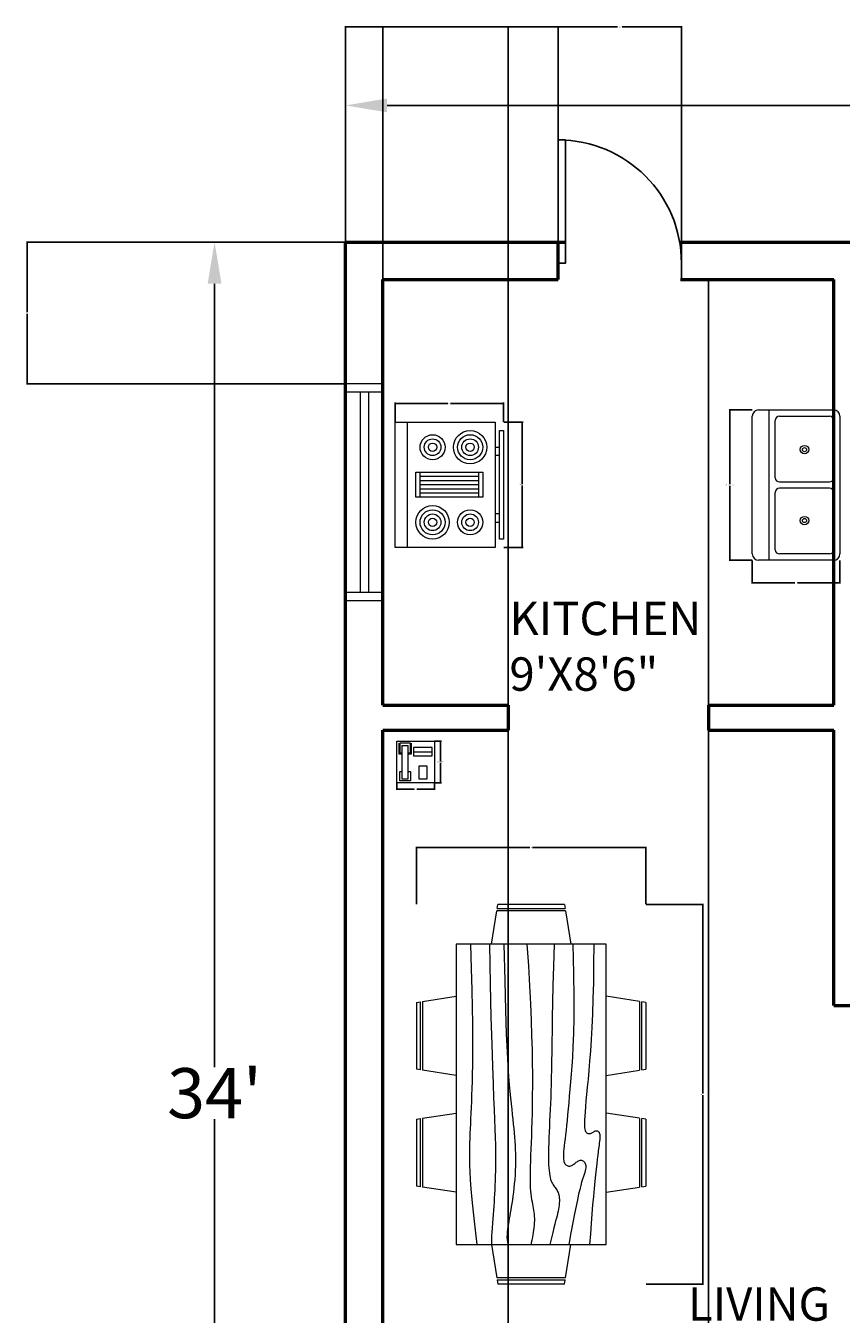
# Model space of a CAD drawing. Units: inches. Extents: x 177 to 602, y 30 to 608.
# Tile 3 of 4: x 177 to 372, y 299 to 608. Entities that reach past the tile are written whole.
import ezdxf

# ---------------------------------------------------------------- set-up
doc = ezdxf.new("R2010")
doc.units = ezdxf.units.IN
doc.header["$MEASUREMENT"] = 0
for name, color, linetype, lineweight in [('A-ANNO-DIMS', 2, 'Continuous', 18), ('A-AREA-IDEN', 7, 'Continuous', 25), ('A-DOOR', 3, 'Continuous', 25), ('A-EQPM', 9, 'Continuous', 18), ('A-FLOR-CASE', 32, 'Continuous', 25), ('A-FLOR-FIXT', 9, 'Continuous', 20), ('A-FURN', 8, 'Continuous', 18), ('A-GLAZ', 4, 'Continuous', 18), ('A-WALL', 7, 'Continuous', 50)]:
    doc.layers.add(name, color=color, linetype=linetype, lineweight=lineweight)
doc.styles.get("Standard").update_dxf_attribs({"font": 'arial.ttf'})
doc.dimstyles.get("Standard").update_dxf_attribs({"dimtxt": 0.18, "dimasz": 0.18, "dimexe": 0.18, "dimexo": 0.0625, "dimgap": 0.09, "dimtad": 0, "dimtih": 1, "dimtoh": 1, "dimdec": 1, "dimzin": 0, "dimdsep": 46, "dimlunit": 4, "dimtxsty": 'Standard', "dimcen": 0.09, "dimadec": 0, "dimazin": 0, "dimtfac": 1, "dimtdec": 1, "dimtofl": 0, "dimtmove": 0, "dimatfit": 3, "dimfxl": 1, "dimtolj": 1, "dimtzin": 0, "dimarcsym": 0})

# ---------------------------------------------------------------- blocks, each defined once
blk = doc.blocks.new('*U2')
for p, q in [((0, 0), (0, -100)), ((750, 0), (750, -100))]:
    blk.add_line(p, q)
blk.add_lwpolyline([(0, 0), (0, 750), (43.75, 750), (43.75, 0)], close=True)
blk.add_arc((0, 0), 750, 0, 90)
blk = doc.blocks.new('Range-Oven - 30 in top')
for p, q in [((0, -3), (30, -3)), ((12, -6), (18, -6)), ((13, -20), (13, -6)), ((14, -6), (14, -20)), ((15, -20), (15, -6)), ((16, -6), (16, -20)), ((17, -20), (17, -6)), ((18, -20), (12, -20)), ((6, -24), (6, -25)), ((8, -25), (8, -24)), ((22, -25), (22, -24)), ((24, -24), (24, -25))]:
    blk.add_line(p, q)
for points in [[(0, -24), (0, 0), (30, 0), (30, -24)], [(12, -21), (12, -5), (18, -5), (18, -21)], [(2, -26), (2, -25), (28, -25), (28, -26)]]:
    blk.add_lwpolyline(points, close=True)
for centre, radius in [((6, -9), 4), ((6, -9), 3), ((24, -9), 3), ((6, -9), 2), ((6, -9), 1), ((24, -9), 2), ((24, -9), 1), ((6, -18), 3), ((24, -18), 4), ((24, -18), 3), ((6, -18), 2), ((6, -18), 1), ((24, -18), 2), ((24, -18), 1)]:
    blk.add_circle(centre, radius)
blk = doc.blocks.new('Sink-double - 36 in top')
for p, q in [((-18, -4), (18, -4)), ((-0.75, -18.5), (-0.75, -6.5)), ((0.75, -6.5), (0.75, -18.5))]:
    blk.add_line(p, q)
for points in [[(-16.5, 0), (16.5, 0)], [(-18, -19.5), (-18, -1.5)], [(18, -1.5), (18, -19.5)], [(-15.5, -5.5), (-1.75, -5.5)], [(1.75, -5.5), (15.5, -5.5)], [(-16.5, -18.5), (-16.5, -6.5)], [(16.5, -6.5), (16.5, -18.5)], [(16.5, -21), (-16.5, -21)], [(-1.75, -19.5), (-15.5, -19.5)], [(15.5, -19.5), (1.75, -19.5)]]:
    blk.add_lwpolyline(points)
for centre, radius in [((-8.5, -12.5), 1), ((-8.5, -12.5), 0.5), ((8.5, -12.5), 1), ((8.5, -12.5), 0.5)]:
    blk.add_circle(centre, radius)
for centre, radius, start, end in [((-16.5, -1.5), 1.5, 90, 180), ((16.5, -1.5), 1.5, 0, 90), ((-15.5, -6.5), 1, 90, 180), ((-1.75, -6.5), 1, 0, 90), ((1.75, -6.5), 1, 90, 180), ((15.5, -6.5), 1, 0, 90), ((-15.5, -18.5), 1, 180, 270), ((-1.75, -18.5), 1, 270, 0), ((1.75, -18.5), 1, 180, 270), ((15.5, -18.5), 1, 270, 0), ((-16.5, -19.5), 1.5, 180, 270), ((16.5, -19.5), 1.5, 270, 0)]:
    blk.add_arc(centre, radius, start, end)
blk = doc.blocks.new('Dining Set - 36 x 72 in.')
for p, q in [((-22.2343, 26.00059), (-23.4847, 17.99762)), ((-22.2304, 26), (-5.7608, 26)), ((-22, 27.5), (-22.1562, 26.50042)), ((-5.8416, 26.5), (-22.1534, 26.5)), ((-22, 27.5), (-6, 27.5)), ((-5.8437, 26.49966), (-6, 27.5)), ((-4.5152, 17.99762), (-5.7655, 25.99926)), ((5.7657, 26.00059), (4.5153, 17.99762)), ((5.7696, 26), (22.2392, 26)), ((6, 27.5), (5.8438, 26.50042)), ((22.1584, 26.5), (5.8466, 26.5)), ((6, 27.5), (22, 27.5)), ((22.1563, 26.49966), (22, 27.5)), ((23.4848, 17.99762), (22.2345, 25.99926)), ((36, 18), (-36, 18)), ((-36, 18), (-36, -18)), ((36, -18), (36, 18)), ((-44.0006, 8.23428), (-35.9976, 9.48474)), ((44.0006, 8.23428), (35.9976, 9.48474)), ((-45.5, 8), (-44.5004, 8.15617)), ((-45.5, 8), (-45.5, -8)), ((-44.5, -8.15843), (-44.5, 8.15338)), ((-44, 8.23041), (-44, -8.23915)), ((44, 8.23041), (44, -8.23915)), ((44.5, -8.15843), (44.5, 8.15338)), ((45.5, 8), (44.5005, 8.15617)), ((45.5, 8), (45.5, -8)), ((-44.4997, -8.15631), (-45.5, -8)), ((-35.9976, -9.48476), (-43.9993, -8.2345)), ((35.9976, -9.48476), (43.9993, -8.2345)), ((44.4997, -8.15631), (45.5, -8)), ((-36, -18), (36, -18)), ((-22.2343, -26.0006), (-23.4847, -17.99762)), ((-4.5152, -17.99762), (-5.7655, -25.99928)), ((5.7657, -26.0006), (4.5153, -17.99762)), ((23.4848, -17.99762), (22.2345, -25.99928)), ((-22.2304, -26), (-5.7608, -26)), ((-22, -27.5), (-22.1562, -26.50044)), ((-5.8416, -26.5), (-22.1534, -26.5)), ((-22, -27.5), (-6, -27.5)), ((-5.8437, -26.49967), (-6, -27.5)), ((5.7696, -26), (22.2392, -26)), ((6, -27.5), (5.8438, -26.50044)), ((22.1584, -26.5), (5.8466, -26.5)), ((6, -27.5), (22, -27.5)), ((22.1563, -26.49967), (22, -27.5))]:
    blk.add_line(p, q)
for points in [[(-36, 15), (-31.1772, 14.97754), (-26.8079, 14.91406), (-22.8538, 14.81543), (-19.276, 14.6875), (-16.0362, 14.53613), (-13.0957, 14.36718), (-10.4159, 14.18652), (-7.9583, 14), (-5.6904, 13.81315), (-3.6035, 13.63021), (-1.6954, 13.45508), (0.0365, 13.29166), (1.5945, 13.14388), (2.9811, 13.01562), (4.1988, 12.9108), (5.25, 12.83333), (6.1393, 12.78613), (6.8802, 12.76823), (7.4883, 12.77767), (7.9792, 12.8125), (8.3685, 12.87077), (8.6719, 12.95052), (8.9049, 13.0498), (9.0833, 13.16666), (9.2205, 13.29899), (9.3216, 13.44401), (9.3895, 13.59879), (9.4271, 13.76041), (9.4373, 13.92594), (9.4232, 14.09245), (9.3875, 14.257), (9.3333, 14.41666), (9.2638, 14.56917), (9.1836, 14.71484), (9.0975, 14.85465), (9.0104, 14.98958), (8.9272, 15.1206), (8.8529, 15.2487), (8.7922, 15.37483), (8.75, 15.5), (8.7305, 15.62467), (8.7344, 15.74739), (8.7617, 15.86621), (8.8125, 15.97916), (8.8867, 16.08431), (8.9844, 16.17968), (9.1055, 16.26334), (9.25, 16.33333), (9.4189, 16.38802), (9.6172, 16.42708), (9.8506, 16.45052), (10.125, 16.45833), (10.4463, 16.45052), (10.8203, 16.42708), (11.2529, 16.38802), (11.75, 16.33333), (12.3184, 16.26318), (12.9694, 16.17838), (13.7151, 16.07991), (14.5677, 15.96875), (15.5395, 15.84586), (16.6426, 15.71224), (17.8893, 15.56884), (19.2917, 15.41666), (20.859, 15.25667), (22.5879, 15.08984), (24.4721, 14.91715), (26.5052, 14.73958), (28.6809, 14.5581), (30.9929, 14.3737), (33.4347, 14.18733), (36, 14)], [(-36, 10), (-28.9766, 10.14274), (-23.1725, 10.20442), (-18.4241, 10.19775), (-14.5677, 10.13541), (-11.4399, 10.03011), (-8.877, 9.89453), (-6.7154, 9.74137), (-4.7917, 9.58333), (-2.9698, 9.43082), (-1.2246, 9.28515), (0.4415, 9.14534), (2.026, 9.01041), (3.5266, 8.87939), (4.9408, 8.7513), (6.266, 8.62516), (7.5, 8.5), (8.6411, 8.37549), (9.6914, 8.2539), (10.6538, 8.13818), (11.5312, 8.03125), (12.3267, 7.93603), (13.043, 7.85547), (13.6831, 7.79248), (14.25, 7.75), (14.7471, 7.7303), (15.1797, 7.73307), (15.5537, 7.75732), (15.875, 7.80208), (16.1494, 7.86637), (16.3828, 7.94922), (16.5811, 8.04964), (16.75, 8.16666), (16.8944, 8.29915), (17.0143, 8.44531), (17.1089, 8.60319), (17.1771, 8.77083), (17.218, 8.94629), (17.2305, 9.1276), (17.2137, 9.31282), (17.1667, 9.5), (17.0895, 9.6875), (16.987, 9.875), (16.8649, 10.0625), (16.7292, 10.25), (16.5856, 10.4375), (16.4401, 10.625), (16.2985, 10.8125), (16.1667, 11), (16.05, 11.18733), (15.9518, 11.3737), (15.8752, 11.5581), (15.8229, 11.73958), (15.798, 11.91715), (15.8034, 12.08984), (15.842, 12.25667), (15.9167, 12.41666), (16.0295, 12.56836), (16.1784, 12.70833), (16.3605, 12.83268), (16.5729, 12.9375), (16.8127, 13.01888), (17.0768, 13.07291), (17.3625, 13.0957), (17.6667, 13.08333), (17.9894, 13.03312), (18.3418, 12.94726), (18.7382, 12.82918), (19.1927, 12.68229), (19.7195, 12.51001), (20.3327, 12.31575), (21.0465, 12.10294), (21.875, 11.875), (22.8357, 11.63354), (23.959, 11.37304), (25.2786, 11.08618), (26.8282, 10.76562), (28.6414, 10.40405), (30.752, 9.99414), (33.1936, 9.52856), (36, 9)], [(-36, 5.5), (-30.7157, 5.3348), (-26.069, 5.20963), (-21.9946, 5.11767), (-18.4271, 5.05208), (-15.3009, 5.00602), (-12.5508, 4.97265), (-10.1112, 4.94515), (-7.9167, 4.91666), (-5.909, 4.88167), (-4.0586, 4.83984), (-2.3429, 4.79215), (-0.7396, 4.73958), (0.7739, 4.6831), (2.22, 4.6237), (3.6213, 4.56233), (5, 4.5), (6.373, 4.43782), (7.7344, 4.3776), (9.0723, 4.32129), (10.375, 4.27083), (11.6309, 4.22819), (12.8281, 4.19531), (13.9551, 4.17415), (15, 4.16666), (15.954, 4.17448), (16.819, 4.19791), (17.6001, 4.23698), (18.3021, 4.29166), (18.9299, 4.36198), (19.4883, 4.44791), (19.9823, 4.54948), (20.4167, 4.66666), (20.7969, 4.79899), (21.1302, 4.94401), (21.4245, 5.09879), (21.6875, 5.26041), (21.9271, 5.42594), (22.1511, 5.59245), (22.3672, 5.757), (22.5834, 5.91666), (22.8065, 6.06868), (23.0404, 6.21093), (23.2879, 6.34147), (23.5521, 6.45833), (23.8358, 6.55957), (24.142, 6.64323), (24.4735, 6.70735), (24.8334, 6.75), (25.2235, 6.76969), (25.642, 6.76692), (26.0858, 6.74267), (26.5521, 6.69791), (27.0379, 6.63362), (27.5404, 6.55078), (28.0565, 6.45036), (28.5834, 6.33333), (29.1242, 6.19987), (29.7071, 6.04687), (30.3661, 5.87044), (31.1354, 5.66666), (32.0493, 5.43164), (33.142, 5.16146), (34.4475, 4.85221), (36, 4.5)], [(-36, -1), (-30.7915, -0.6591), (-26.0195, -0.38216), (-21.6519, -0.16284), (-17.6563, 0.00521), (-14.0005, 0.12833), (-10.6523, 0.21289), (-7.5796, 0.26522), (-4.75, 0.29166), (-2.134, 0.29793), (0.2878, 0.28711), (2.5317, 0.26163), (4.6146, 0.22396), (6.5529, 0.17651), (8.3633, 0.12174), (10.0623, 0.06209), (11.6667, 0), (13.1899, -0.06201), (14.6341, -0.1211), (15.9982, -0.17432), (17.2813, -0.21875), (18.4823, -0.25147), (19.6003, -0.26953), (20.6343, -0.27002), (21.5834, -0.25), (22.4481, -0.20768), (23.2357, -0.14584), (23.9549, -0.06836), (24.6146, 0.02083), (25.2235, 0.11784), (25.7904, 0.21875), (26.3241, 0.31966), (26.8334, 0.41666), (27.3265, 0.50618), (27.8099, 0.58593), (28.2894, 0.65397), (28.7709, 0.70833), (29.2601, 0.74707), (29.763, 0.76823), (30.2855, 0.76985), (30.8334, 0.75), (31.4088, 0.70784), (31.9994, 0.64713), (32.589, 0.57275), (33.1615, 0.48958), (33.7008, 0.4025), (34.1908, 0.3164), (34.6153, 0.23616), (34.9584, 0.16666), (35.2099, 0.11165), (35.3848, 0.07031), (35.504, 0.04069), (35.5886, 0.02083), (35.6594, 0.00879), (35.7377, 0.0026), (35.8442, 0.00032), (36, 0)], [(-36, -6.5), (-27.1843, -6.31267), (-20.084, -6.1263), (-14.469, -5.9419), (-10.1094, -5.76042), (-6.7752, -5.58285), (-4.2363, -5.41016), (-2.2629, -5.24333), (-0.625, -5.08334), (0.8708, -4.93099), (2.2715, -4.78646), (3.5872, -4.64974), (4.8281, -4.52084), (6.0046, -4.39974), (7.127, -4.28646), (8.2053, -4.18099), (9.25, -4.08334), (10.2705, -3.99382), (11.2734, -3.91407), (12.2647, -3.84603), (13.25, -3.79167), (14.2354, -3.75293), (15.2266, -3.73177), (16.2295, -3.73015), (17.25, -3.75), (18.2912, -3.79248), (19.3451, -3.85547), (20.4009, -3.93604), (21.4479, -4.03125), (22.4754, -4.13819), (23.4727, -4.25391), (24.4289, -4.37549), (25.3334, -4.5), (26.1785, -4.62492), (26.9694, -4.74935), (27.7145, -4.87281), (28.4219, -4.99479), (29.1, -5.11483), (29.7572, -5.23242), (30.4016, -5.34709), (31.0417, -5.45834), (31.6837, -5.56437), (32.3262, -5.65821), (32.9658, -5.73153), (33.599, -5.77604), (34.2224, -5.78345), (34.8327, -5.74545), (35.4264, -5.65373), (36, -5.5)], [(-36, -10), (-26.4022, -9.81299), (-18.4675, -9.62891), (-11.9839, -9.45069), (-6.7396, -9.28125), (-2.5226, -9.12354), (0.8789, -8.98047), (3.6769, -8.85498), (6.0833, -8.75), (8.2767, -8.66765), (10.3021, -8.60677), (12.1712, -8.56543), (13.8958, -8.54167), (15.4876, -8.53353), (16.9583, -8.53907), (18.3197, -8.55632), (19.5834, -8.58334), (20.7616, -8.61841), (21.8685, -8.66081), (22.9188, -8.71004), (23.9271, -8.76563), (24.9081, -8.82707), (25.8763, -8.89388), (26.8465, -8.96558), (27.8334, -9.04167), (28.8474, -9.12118), (29.8828, -9.20117), (30.93, -9.27824), (31.9792, -9.34896), (33.0205, -9.40991), (34.0443, -9.45768), (35.0407, -9.48885), (36, -9.5)], [(-36, -14.5), (-30.0881, -14.33513), (-25.0332, -14.21224), (-20.7312, -14.12647), (-17.0781, -14.07292), (-13.97, -14.04671), (-11.3027, -14.04297), (-8.9724, -14.05681), (-6.875, -14.08334), (-4.9224, -14.11833), (-3.0905, -14.16016), (-1.3709, -14.20785), (0.2448, -14.26042), (1.7647, -14.3169), (3.1973, -14.3763), (4.5507, -14.43767), (5.8333, -14.5), (7.0554, -14.5621), (8.235, -14.62175), (9.3922, -14.67652), (10.5469, -14.72396), (11.7192, -14.76164), (12.929, -14.78711), (14.1965, -14.79794), (15.5417, -14.79167), (16.9933, -14.76424), (18.6152, -14.70508), (20.4804, -14.60197), (22.6615, -14.44271), (25.2312, -14.21509), (28.2624, -13.9069), (31.8277, -13.50594), (36, -13)]]:
    blk.add_lwpolyline(points)
blk = doc.blocks.new('Phone - Desk')
for p, q in [((-4.5, -5), (-4.5, 5)), ((-4.5, 5), (4.5, 5)), ((-4, 4.5), (-4, 2)), ((-3.75, 4.5), (-3.75, 2.25)), ((-1.25, 4.5), (-3.75, 4.5)), ((-3.25, 4), (-3.25, -4)), ((-3.25, 4), (-1.75, 4)), ((-1.75, -4), (-1.75, 4)), ((-1.25, 2.25), (-1.25, 4.5)), ((-1, 2), (-1, 4.5)), ((4, 3.5), (-0.5, 3.5)), ((-0.5, 3.5), (-0.5, 1.5)), ((4, 1.5), (4, 3.5)), ((4.5, 5), (4.5, -5)), ((-4, 2), (-3.25, 2)), ((-3.75, 2.25), (-3.25, 2.25)), ((-1.75, 2.25), (-1.25, 2.25)), ((-1.75, 2), (-1, 2)), ((-0.5, 2.5), (4, 2.5)), ((-0.5, 1.5), (4, 1.5)), ((-3.75, -2.25), (-3.25, -2.25)), ((-3.75, -4.5), (-3.75, -2.25)), ((-1.75, -2.25), (-1.25, -2.25)), ((-1.25, -2.25), (-1.25, -4.5)), ((2.75, -1), (0.75, -1)), ((0.75, -1), (0.75, -4)), ((2.75, -4), (2.75, -1)), ((4.5, -5), (-4.5, -5)), ((-1.25, -4.5), (-3.75, -4.5)), ((-3.25, -4), (-1.75, -4)), ((0.75, -4), (2.75, -4))]:
    blk.add_line(p, q)
blk = doc.blocks.new('*D32')
at = {"layer": 'A-ANNO-DIMS', "color": 0, "lineweight": -2, "transparency": 16777216}
for p, q in [((253.34, 556.2), (253.34, 589.06)), ((263.34, 588.88), (398.96, 588.88)), ((555.34, 588.88), (419.71, 588.88)), ((565.34, 556.2), (565.34, 589.06))]:
    blk.add_line(p, q, dxfattribs=at)
at = {"layer": 'A-ANNO-DIMS', "color": 0, "transparency": 16777216}
for points in [[(263.34, 590.55), (263.34, 587.22), (253.34, 588.88)], [(555.34, 590.55), (555.34, 587.22), (565.34, 588.88)]]:
    blk.add_solid(points, dxfattribs=at)
at = {"layer": 'Defpoints', "color": 0, "transparency": 16777216}
for p in [(565.34, 588.88), (253.34, 556.14), (565.34, 556.14)]:
    blk.add_point(p, dxfattribs=at)
at = {"layer": 'A-ANNO-DIMS', "color": 0, "transparency": 16777216, "insert": (409.34, 588.88), "char_height": 12, "attachment_point": 5}
blk.add_mtext("\\A1;26'", dxfattribs=at)
blk = doc.blocks.new('*D33')
at = {"layer": 'A-ANNO-DIMS', "color": 0, "lineweight": -2, "transparency": 16777216}
for p, q in [((253.28, 556.14), (221.81, 556.14)), ((221.99, 546.14), (221.99, 358.36)), ((221.99, 158.14), (221.99, 345.92)), ((253.28, 148.14), (221.81, 148.14))]:
    blk.add_line(p, q, dxfattribs=at)
at = {"layer": 'A-ANNO-DIMS', "color": 0, "transparency": 16777216}
for points in [[(220.33, 546.14), (223.66, 546.14), (221.99, 556.14)], [(220.33, 158.14), (223.66, 158.14), (221.99, 148.14)]]:
    blk.add_solid(points, dxfattribs=at)
at = {"layer": 'Defpoints', "color": 0, "transparency": 16777216}
for p in [(221.99, 556.14), (253.34, 556.14), (253.34, 148.14)]:
    blk.add_point(p, dxfattribs=at)
at = {"layer": 'A-ANNO-DIMS', "color": 0, "transparency": 16777216, "insert": (221.99, 352.14), "char_height": 12, "attachment_point": 5}
blk.add_mtext("\\A1;34'", dxfattribs=at)
blk = doc.blocks.new('WIN-48IN')
for p, q in [((9, 52), (0, 52)), ((9, 50), (0, 50)), ((3.5, 50), (3.5, 2)), ((5.5, 50), (5.5, 2)), ((9, 2), (0, 2)), ((9, 0), (0, 0))]:
    blk.add_line(p, q)
blk = doc.blocks.new('*D43')
at = {"layer": 'A-ANNO-DIMS', "color": 0, "lineweight": -2, "transparency": 16777216}
for p, q in [((291.29, 512.96), (295.91, 512.96)), ((295.73, 512.78), (295.73, 498.14)), ((295.73, 483.14), (295.73, 497.77)), ((291.29, 482.96), (295.91, 482.96))]:
    blk.add_line(p, q, dxfattribs=at)
at = {"layer": 'A-ANNO-DIMS', "color": 0, "transparency": 16777216}
for points in [[(295.7, 512.78), (295.76, 512.78), (295.73, 512.96)], [(295.7, 483.14), (295.76, 483.14), (295.73, 482.96)]]:
    blk.add_solid(points, dxfattribs=at)
at = {"layer": 'Defpoints', "color": 0, "transparency": 16777216}
for p in [(291.23, 512.96), (295.73, 512.96), (291.23, 482.96)]:
    blk.add_point(p, dxfattribs=at)
at = {"layer": 'A-ANNO-DIMS', "color": 0, "transparency": 16777216, "insert": (295.73, 497.96), "char_height": 0.18, "attachment_point": 5}
blk.add_mtext('\\A1;RANGE 2\'-6"', dxfattribs=at)
blk = doc.blocks.new('*D44')
at = {"layer": 'A-ANNO-DIMS', "color": 0, "lineweight": -2, "transparency": 16777216}
for p, q in [((265.23, 513.02), (265.23, 517.64)), ((265.41, 517.46), (277.9, 517.46)), ((291.05, 517.46), (278.56, 517.46)), ((291.23, 513.02), (291.23, 517.64))]:
    blk.add_line(p, q, dxfattribs=at)
at = {"layer": 'A-ANNO-DIMS', "color": 0, "transparency": 16777216}
for points in [[(265.41, 517.49), (265.41, 517.43), (265.23, 517.46)], [(291.05, 517.49), (291.05, 517.43), (291.23, 517.46)]]:
    blk.add_solid(points, dxfattribs=at)
at = {"layer": 'Defpoints', "color": 0, "transparency": 16777216}
for p in [(265.23, 517.46), (265.23, 512.96), (291.23, 512.96)]:
    blk.add_point(p, dxfattribs=at)
at = {"layer": 'A-ANNO-DIMS', "color": 0, "transparency": 16777216, "insert": (278.23, 517.46), "char_height": 0.18, "attachment_point": 5}
blk.add_mtext('\\A1;2\'-2"', dxfattribs=at)
blk = doc.blocks.new('*D45')
at = {"layer": 'A-ANNO-DIMS', "color": 0, "lineweight": -2, "transparency": 16777216}
for p, q in [((350.78, 515.89), (345.26, 515.89)), ((345.44, 515.71), (345.44, 498.07)), ((345.44, 480.07), (345.44, 497.7)), ((350.78, 479.89), (345.26, 479.89))]:
    blk.add_line(p, q, dxfattribs=at)
at = {"layer": 'A-ANNO-DIMS', "color": 0, "transparency": 16777216}
for points in [[(345.41, 515.71), (345.47, 515.71), (345.44, 515.89)], [(345.41, 480.07), (345.47, 480.07), (345.44, 479.89)]]:
    blk.add_solid(points, dxfattribs=at)
at = {"layer": 'Defpoints', "color": 0, "transparency": 16777216}
for p in [(345.44, 515.89), (350.84, 515.89), (350.84, 479.89)]:
    blk.add_point(p, dxfattribs=at)
at = {"layer": 'A-ANNO-DIMS', "color": 0, "transparency": 16777216, "insert": (345.44, 497.89), "char_height": 0.18, "attachment_point": 5}
blk.add_mtext('\\A1;DOUBLE SINK 3\'-0"', dxfattribs=at)
blk = doc.blocks.new('*D46')
at = {"layer": 'A-ANNO-DIMS', "color": 0, "lineweight": -2, "transparency": 16777216}
for p, q in [((350.84, 479.82), (350.84, 474.31)), ((371.84, 479.82), (371.84, 474.31)), ((351.02, 474.49), (361.02, 474.49)), ((371.66, 474.49), (361.66, 474.49))]:
    blk.add_line(p, q, dxfattribs=at)
at = {"layer": 'A-ANNO-DIMS', "color": 0, "transparency": 16777216}
for points in [[(351.02, 474.52), (351.02, 474.46), (350.84, 474.49)], [(371.66, 474.52), (371.66, 474.46), (371.84, 474.49)]]:
    blk.add_solid(points, dxfattribs=at)
at = {"layer": 'Defpoints', "color": 0, "transparency": 16777216}
for p in [(350.84, 479.89), (371.84, 479.89), (350.84, 474.49)]:
    blk.add_point(p, dxfattribs=at)
at = {"layer": 'A-ANNO-DIMS', "color": 0, "transparency": 16777216, "insert": (361.34, 474.49), "char_height": 0.18, "attachment_point": 5}
blk.add_mtext('\\A1;1\'-9"', dxfattribs=at)
blk = doc.blocks.new('*D47')
at = {"layer": 'A-ANNO-DIMS', "color": 0, "lineweight": -2, "transparency": 16777216}
for p, q in [((325.41, 397.38), (339.17, 397.38)), ((338.99, 397.2), (338.99, 352.06)), ((338.99, 306.56), (338.99, 351.69)), ((325.41, 306.38), (339.17, 306.38))]:
    blk.add_line(p, q, dxfattribs=at)
at = {"layer": 'A-ANNO-DIMS', "color": 0, "transparency": 16777216}
for points in [[(338.96, 397.2), (339.02, 397.2), (338.99, 397.38)], [(338.96, 306.56), (339.02, 306.56), (338.99, 306.38)]]:
    blk.add_solid(points, dxfattribs=at)
at = {"layer": 'Defpoints', "color": 0, "transparency": 16777216}
for p in [(325.34, 397.38), (325.34, 306.38), (338.99, 306.38)]:
    blk.add_point(p, dxfattribs=at)
at = {"layer": 'A-ANNO-DIMS', "color": 0, "transparency": 16777216, "insert": (338.99, 351.88), "char_height": 0.18, "attachment_point": 5}
blk.add_mtext('\\A1;DINING SET 7\'-7"', dxfattribs=at)
blk = doc.blocks.new('*D48')
at = {"layer": 'A-ANNO-DIMS', "color": 0, "lineweight": -2, "transparency": 16777216}
for p, q in [((270.34, 397.44), (270.34, 411.21)), ((270.52, 411.03), (297.51, 411.03)), ((325.16, 411.03), (298.18, 411.03)), ((325.34, 397.44), (325.34, 411.21))]:
    blk.add_line(p, q, dxfattribs=at)
at = {"layer": 'A-ANNO-DIMS', "color": 0, "transparency": 16777216}
for points in [[(270.52, 411.06), (270.52, 411), (270.34, 411.03)], [(325.16, 411.06), (325.16, 411), (325.34, 411.03)]]:
    blk.add_solid(points, dxfattribs=at)
at = {"layer": 'Defpoints', "color": 0, "transparency": 16777216}
for p in [(325.34, 411.03), (270.34, 397.38), (325.34, 397.38)]:
    blk.add_point(p, dxfattribs=at)
at = {"layer": 'A-ANNO-DIMS', "color": 0, "transparency": 16777216, "insert": (297.84, 411.03), "char_height": 0.18, "attachment_point": 5}
blk.add_mtext('\\A1;4\'-7"', dxfattribs=at)
blk = doc.blocks.new('*D61')
at = {"layer": 'A-ANNO-DIMS', "color": 0, "lineweight": -2, "transparency": 16777216}
for p, q in [((274.71, 436.49), (276.33, 436.49)), ((276.15, 436.31), (276.15, 431.67)), ((276.15, 426.67), (276.15, 431.3)), ((274.71, 426.49), (276.33, 426.49))]:
    blk.add_line(p, q, dxfattribs=at)
at = {"layer": 'A-ANNO-DIMS', "color": 0, "transparency": 16777216}
for points in [[(276.12, 436.31), (276.18, 436.31), (276.15, 436.49)], [(276.12, 426.67), (276.18, 426.67), (276.15, 426.49)]]:
    blk.add_solid(points, dxfattribs=at)
at = {"layer": 'Defpoints', "color": 0, "transparency": 16777216}
for p in [(274.65, 436.49), (276.15, 436.49), (274.65, 426.49)]:
    blk.add_point(p, dxfattribs=at)
at = {"layer": 'A-ANNO-DIMS', "color": 0, "transparency": 16777216, "insert": (276.15, 431.49), "char_height": 0.18, "attachment_point": 5}
blk.add_mtext('\\A1;PHONE 0\'-10"', dxfattribs=at)
blk = doc.blocks.new('*D62')
at = {"layer": 'A-ANNO-DIMS', "color": 0, "lineweight": -2, "transparency": 16777216}
for p, q in [((265.65, 426.42), (265.65, 424.81)), ((274.65, 426.42), (274.65, 424.81)), ((265.83, 424.99), (269.82, 424.99)), ((274.47, 424.99), (270.48, 424.99))]:
    blk.add_line(p, q, dxfattribs=at)
at = {"layer": 'A-ANNO-DIMS', "color": 0, "transparency": 16777216}
for points in [[(265.83, 425.02), (265.83, 424.96), (265.65, 424.99)], [(274.47, 425.02), (274.47, 424.96), (274.65, 424.99)]]:
    blk.add_solid(points, dxfattribs=at)
at = {"layer": 'Defpoints', "color": 0, "transparency": 16777216}
for p in [(265.65, 426.49), (274.65, 426.49), (274.65, 424.99)]:
    blk.add_point(p, dxfattribs=at)
at = {"layer": 'A-ANNO-DIMS', "color": 0, "transparency": 16777216, "insert": (270.15, 424.99), "char_height": 0.18, "attachment_point": 5}
blk.add_mtext('\\A1;0\'-9"', dxfattribs=at)
blk = doc.blocks.new('*D75')
at = {"layer": 'A-ANNO-DIMS', "color": 0, "lineweight": -2, "transparency": 16777216}
for p, q in [((253.34, 556.2), (253.34, 607.88)), ((253.52, 607.7), (278.51, 607.7)), ((304.16, 607.7), (279.17, 607.7)), ((304.34, 556.2), (304.34, 607.88))]:
    blk.add_line(p, q, dxfattribs=at)
at = {"layer": 'A-ANNO-DIMS', "color": 0, "transparency": 16777216}
for points in [[(253.52, 607.73), (253.52, 607.67), (253.34, 607.7)], [(304.16, 607.73), (304.16, 607.67), (304.34, 607.7)]]:
    blk.add_solid(points, dxfattribs=at)
at = {"layer": 'Defpoints', "color": 0, "transparency": 16777216}
for p in [(304.34, 607.7), (253.34, 556.14), (304.34, 556.14)]:
    blk.add_point(p, dxfattribs=at)
at = {"layer": 'A-ANNO-DIMS', "color": 0, "transparency": 16777216, "insert": (278.84, 607.7), "char_height": 0.18, "attachment_point": 5}
blk.add_mtext('\\A1;4\'-3"', dxfattribs=at)
blk = doc.blocks.new('*D76')
at = {"layer": 'A-ANNO-DIMS', "color": 0, "lineweight": -2, "transparency": 16777216}
for p, q in [((304.34, 547.2), (304.34, 607.88)), ((304.52, 607.7), (318.56, 607.7)), ((333.69, 607.7), (319.64, 607.7)), ((333.87, 547.2), (333.87, 607.88))]:
    blk.add_line(p, q, dxfattribs=at)
at = {"layer": 'A-ANNO-DIMS', "color": 0, "transparency": 16777216}
for points in [[(304.52, 607.73), (304.52, 607.67), (304.34, 607.7)], [(333.69, 607.73), (333.69, 607.67), (333.87, 607.7)]]:
    blk.add_solid(points, dxfattribs=at)
at = {"layer": 'Defpoints', "color": 0, "transparency": 16777216}
for p in [(333.87, 607.7), (304.34, 547.14), (333.87, 547.14)]:
    blk.add_point(p, dxfattribs=at)
at = {"layer": 'A-ANNO-DIMS', "color": 0, "transparency": 16777216, "insert": (319.1, 607.7), "char_height": 0.18, "attachment_point": 5}
blk.add_mtext('\\A1;2\'-5 1/2"', dxfattribs=at)
blk = doc.blocks.new('*D81')
at = {"layer": 'A-ANNO-DIMS', "color": 0, "lineweight": -2, "transparency": 16777216}
for p, q in [((253.28, 556.14), (176.92, 556.14)), ((177.1, 555.96), (177.1, 539.32)), ((177.1, 522.32), (177.1, 538.96)), ((253.28, 522.14), (176.92, 522.14))]:
    blk.add_line(p, q, dxfattribs=at)
at = {"layer": 'A-ANNO-DIMS', "color": 0, "transparency": 16777216}
for points in [[(177.07, 555.96), (177.13, 555.96), (177.1, 556.14)], [(177.07, 522.32), (177.13, 522.32), (177.1, 522.14)]]:
    blk.add_solid(points, dxfattribs=at)
at = {"layer": 'Defpoints', "color": 0, "transparency": 16777216}
for p in [(177.1, 556.14), (253.34, 556.14), (253.34, 522.14)]:
    blk.add_point(p, dxfattribs=at)
at = {"layer": 'A-ANNO-DIMS', "color": 0, "transparency": 16777216, "insert": (177.1, 539.14), "char_height": 0.18, "attachment_point": 5}
blk.add_mtext('\\A1;2\'-10"', dxfattribs=at)
blk = doc.blocks.new('*D85')
at = {"layer": 'A-ANNO-DIMS', "color": 0, "lineweight": -2, "transparency": 16777216}
for p, q in [((292.34, 445.07), (292.34, 30.54)), ((340.34, 445.07), (340.34, 30.54)), ((292.52, 30.72), (316.01, 30.72)), ((340.16, 30.72), (316.67, 30.72))]:
    blk.add_line(p, q, dxfattribs=at)
at = {"layer": 'A-ANNO-DIMS', "color": 0, "transparency": 16777216}
for points in [[(292.52, 30.75), (292.52, 30.69), (292.34, 30.72)], [(340.16, 30.75), (340.16, 30.69), (340.34, 30.72)]]:
    blk.add_solid(points, dxfattribs=at)
at = {"layer": 'Defpoints', "color": 0, "transparency": 16777216}
for p in [(292.34, 445.14), (340.34, 445.14), (340.34, 30.72)]:
    blk.add_point(p, dxfattribs=at)
at = {"layer": 'A-ANNO-DIMS', "color": 0, "transparency": 16777216, "insert": (316.34, 30.72), "char_height": 0.18, "attachment_point": 5}
blk.add_mtext('\\A1;4\'-0"', dxfattribs=at)
blk = doc.blocks.new('*D86')
at = {"layer": 'A-ANNO-DIMS', "color": 0, "lineweight": -2, "transparency": 16777216}
for p, q in [((262.34, 547.2), (262.34, 607.88)), ((262.52, 607.7), (277.01, 607.7)), ((292.16, 607.7), (277.67, 607.7)), ((292.34, 547.2), (292.34, 607.88))]:
    blk.add_line(p, q, dxfattribs=at)
at = {"layer": 'A-ANNO-DIMS', "color": 0, "transparency": 16777216}
for points in [[(262.52, 607.73), (262.52, 607.67), (262.34, 607.7)], [(292.16, 607.73), (292.16, 607.67), (292.34, 607.7)]]:
    blk.add_solid(points, dxfattribs=at)
at = {"layer": 'Defpoints', "color": 0, "transparency": 16777216}
for p in [(292.34, 607.7), (262.34, 547.14), (292.34, 547.14)]:
    blk.add_point(p, dxfattribs=at)
at = {"layer": 'A-ANNO-DIMS', "color": 0, "transparency": 16777216, "insert": (277.34, 607.7), "char_height": 0.18, "attachment_point": 5}
blk.add_mtext('\\A1;2\'-6"', dxfattribs=at)

msp = doc.modelspace()

# ---------------------------------------------------------------- linework, layer by layer
at = {"layer": 'A-FLOR-CASE'}
for p, q in [((292.34, 445.14), (292.34, 547.14)), ((340.34, 445.14), (340.34, 547.14))]:
    msp.add_line(p, q, dxfattribs=at)
at = {"layer": 'A-WALL'}
for p, q in [((253.34, 556.14), (306.06, 556.14)), ((253.34, 148.14), (253.34, 556.14)), ((304.34, 547.14), (304.34, 556.14)), ((333.43, 556.14), (565.34, 556.14)), ((262.34, 547.14), (304.34, 547.14)), ((262.34, 445.14), (262.34, 547.14)), ((333.6, 547.14), (370.34, 547.14)), ((370.34, 445.14), (370.34, 547.14)), ((262.34, 445.14), (292.34, 445.14)), ((292.34, 445.14), (292.34, 439.14)), ((340.34, 445.14), (340.34, 439.14)), ((340.34, 445.14), (370.34, 445.14)), ((262.34, 157.14), (262.34, 439.14)), ((262.34, 439.14), (292.34, 439.14)), ((340.34, 439.14), (370.34, 439.14)), ((370.34, 373.14), (370.34, 439.14)), ((370.34, 373.14), (401.08, 373.14))]:
    msp.add_line(p, q, dxfattribs=at)

# ---------------------------------------------------------------- block references
at = {"layer": 'A-DOOR', "xscale": 0.0393700787401575, "yscale": 0.0393700787401575, "zscale": 0.0393700787401575}
msp.add_blockref('*U2', (304.34, 551.07), dxfattribs=at)
at = {"layer": 'A-EQPM', "rotation": 90}
msp.add_blockref('Range-Oven - 30 in top', (265.23, 482.96), dxfattribs=at)
at = {"layer": 'A-EQPM'}
msp.add_blockref('Phone - Desk', (270.15, 431.49), dxfattribs=at)
at = {"layer": 'A-FLOR-FIXT', "rotation": 90}
msp.add_blockref('Sink-double - 36 in top', (350.84, 497.89), dxfattribs=at)
at = {"layer": 'A-FURN', "rotation": 270}
msp.add_blockref('Dining Set - 36 x 72 in.', (297.84, 351.88), dxfattribs=at)
at = {"layer": 'A-GLAZ'}
msp.add_blockref('WIN-48IN', (253.34, 470.14), dxfattribs=at)

# ---------------------------------------------------------------- texts
at = {"layer": 'A-AREA-IDEN', "char_height": 8, "attachment_point": 1}
for s, insert in [('KITCHEN\\P9\'X8\'6"', (292.63, 469.93)), ('  LIVING\\P19\'6"X12\'1"', (330.54, 305.6))]:
    msp.add_mtext_dynamic_manual_height_columns(s, width=62.7486, gutter_width=1, heights=[0], dxfattribs=dict(at, insert=insert))

# ---------------------------------------------------------------- dimensions: what is measured, and where the dimension line sits
at = {"layer": 'A-ANNO-DIMS'}
for base, p1, p2, override, picture, middle in [((304.34, 607.7), (253.34, 556.14), (304.34, 556.14), {"dimdec": 1, "dimlfac": 1, "dimrnd": 0, "dimzin": 1, "dimdsep": 46, "dimlunit": 4, "dimfrac": 2}, '*D75', (278.84, 607.7)), ((292.34, 607.7), (262.34, 547.14), (292.34, 547.14), {"dimdec": 1, "dimlfac": 1, "dimrnd": 0, "dimzin": 1, "dimdsep": 46, "dimlunit": 4, "dimfrac": 2}, '*D86', (277.34, 607.7)), ((333.87, 607.7), (304.34, 547.14), (333.87, 547.14), {"dimdec": 1, "dimlfac": 1, "dimrnd": 0, "dimzin": 1, "dimdsep": 46, "dimlunit": 4, "dimfrac": 2}, '*D76', (319.1, 607.7)), ((565.34, 588.88), (253.34, 556.14), (565.34, 556.14), {"dimtxt": 12, "dimasz": 10, "dimclrd": 0, "dimclre": 0, "dimclrt": 0}, '*D32', (409.34, 588.88)), ((340.34, 30.72), (292.34, 445.14), (340.34, 445.14), {"dimdec": 1, "dimlfac": 1, "dimrnd": 0, "dimzin": 1, "dimdsep": 46, "dimlunit": 4, "dimfrac": 2}, '*D85', (316.34, 30.72)), ((274.65, 424.99), (265.65, 426.49), (274.65, 426.49), {"dimdec": 1, "dimlfac": 1, "dimrnd": 0, "dimzin": 1, "dimdsep": 46, "dimlunit": 4, "dimfrac": 2}, '*D62', (270.15, 424.99)), ((325.34, 411.03), (270.34, 397.38), (325.34, 397.38), {"dimdec": 1, "dimlfac": 1, "dimrnd": 0, "dimzin": 1, "dimdsep": 46, "dimlunit": 4, "dimfrac": 2}, '*D48', (297.84, 411.03))]:
    dim = msp.add_linear_dim(base=base, p1=p1, p2=p2, dimstyle='Standard', override=override, dxfattribs=at)
    dim.commit()
    dim.dimension.update_dxf_attribs({"geometry": picture, "text_midpoint": middle})
for base, p1, p2, angle, override, picture, middle in [((177.1, 556.14), (253.34, 522.14), (253.34, 556.14), 90, {"dimdec": 1, "dimlfac": 1, "dimrnd": 0, "dimzin": 1, "dimdsep": 46, "dimlunit": 4, "dimfrac": 2}, '*D81', (177.1, 539.14)), ((221.99, 556.14), (253.34, 148.14), (253.34, 556.14), 90, {"dimtxt": 12, "dimasz": 10, "dimclrd": 0, "dimclre": 0, "dimclrt": 0}, '*D33', (221.99, 352.14)), ((265.23, 517.46), (291.23, 512.96), (265.23, 512.96), 180, {"dimdec": 1, "dimlfac": 1, "dimrnd": 0, "dimzin": 1, "dimdsep": 46, "dimlunit": 4, "dimfrac": 2}, '*D44', (278.23, 517.46)), ((350.84, 474.49), (371.84, 479.89), (350.84, 479.89), 180, {"dimdec": 1, "dimlfac": 1, "dimrnd": 0, "dimzin": 1, "dimdsep": 46, "dimlunit": 4, "dimfrac": 2}, '*D46', (361.34, 474.49))]:
    dim = msp.add_linear_dim(base=base, p1=p1, p2=p2, angle=angle, dimstyle='Standard', override=override, dxfattribs=at)
    dim.commit()
    dim.dimension.update_dxf_attribs({"geometry": picture, "text_midpoint": middle})
for base, p1, p2, angle, text, picture, middle in [((345.44, 515.89), (350.84, 479.89), (350.84, 515.89), 90, 'DOUBLE SINK <>', '*D45', (345.44, 497.89)), ((295.73, 512.96), (291.23, 482.96), (291.23, 512.96), 90, 'RANGE <>', '*D43', (295.73, 497.96)), ((276.15, 436.49), (274.65, 426.49), (274.65, 436.49), 90, 'PHONE <>', '*D61', (276.15, 431.49)), ((338.99, 306.38), (325.34, 397.38), (325.34, 306.38), 270, 'DINING SET <>', '*D47', (338.99, 351.88))]:
    dim = msp.add_linear_dim(base=base, p1=p1, p2=p2, angle=angle, text=text, dimstyle='Standard', override={"dimdec": 1, "dimlfac": 1, "dimrnd": 0, "dimzin": 1, "dimdsep": 46, "dimlunit": 4, "dimfrac": 2}, dxfattribs=at)
    dim.commit()
    dim.dimension.update_dxf_attribs({"geometry": picture, "text_midpoint": middle})

doc.saveas('drawing.dxf')
